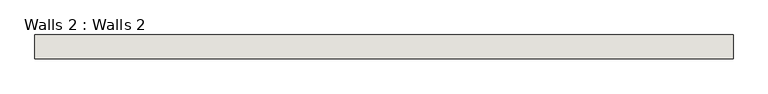
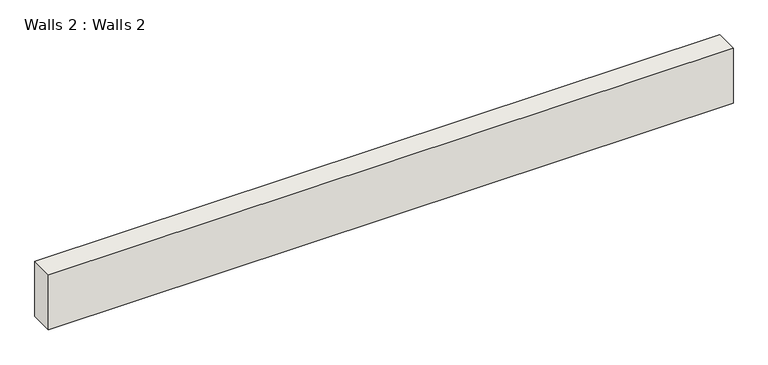
"""IFC4 building model written with IfcOpenShell, lengths in millimetres: wall geometry, Walls 2 : Walls 2."""

from ifc_helpers import new_model, si_unit, frame, origin, place, context, project, spatial, polyline, outline, extrude, source, transform, mapped, element, save


def walls_2_walls_2_1c393272(model_context):
    return source(origin(), model_context, "Body", "SweptSolid", [
        extrude(outline(polyline([(-4767.330251, 2572.873096), (-13671.3981295, 2572.873096), (-13671.3981295, 2877.673096), (-4767.330251, 2877.673096), (-4767.330251, 2572.873096)])), frame((0.0, 0.0, 3239.9410058), z_axis=(0.0, 0.0, 1.0), x_axis=(1.0, 0.0, 0.0)), (0.0, 0.0, 1.0), 757.7613553),
    ])


if __name__ == "__main__":
    model = new_model("IFC4")
    model_context = context("Model", 3, world=origin())
    ifc_project = project(units=[si_unit("LENGTHUNIT", "METRE", prefix="MILLI")], contexts=[model_context])
    site = spatial("IfcSite", under=ifc_project)
    building = spatial("IfcBuilding", under=site)
    placement = place(None, origin())
    walls_2_walls_2_shape = walls_2_walls_2_1c393272(model_context)
    element("IfcWall", 1, ObjectType="Walls 2 : Walls 2", at=placement, inside=building, context=model_context, shape_type="MappedRepresentation", body=[
        mapped(walls_2_walls_2_shape, transform((0.0, 0.0, 0.0), x_axis=(1.0, 0.0, 0.0), y_axis=(0.0, 1.0, 0.0), z_axis=(0.0, 0.0, 1.0))),
    ])
    save(model, "model.ifc")

# Revit data of these elements
# Element 1 (IfcWall, "Walls 2 : Walls 2")
#   Materials on its faces: "Default Wall"
# Materials
#   "Default Wall": colour RGB 128 128 128, transparency 0
